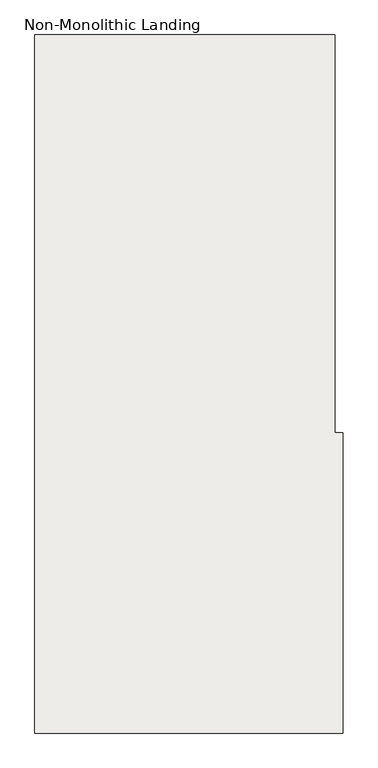
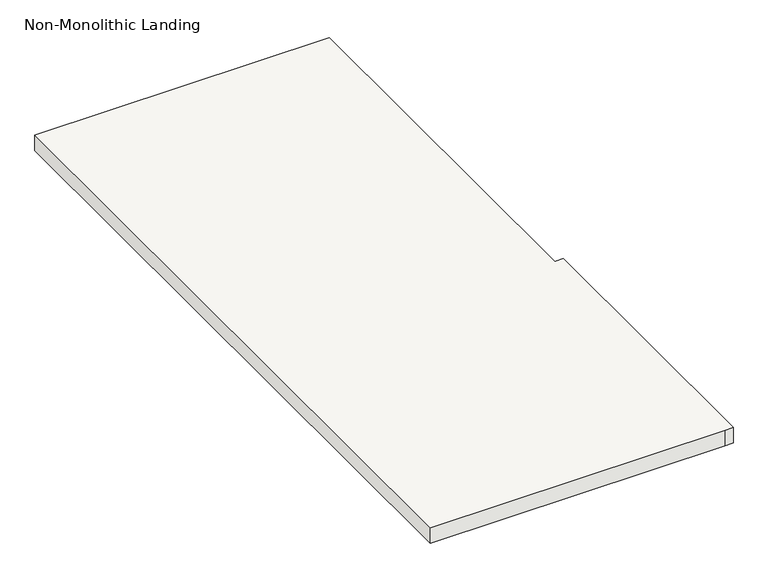
"""IFC4 building model written with IfcOpenShell, lengths in millimetres: slab geometry, Non-Monolithic Landing."""

from ifc_helpers import new_model, si_unit, origin, place, context, project, spatial, faceted_brep, source, transform, mapped, element, save


def non_monolithic_landing_459b2879(model_context):
    return source(origin(), model_context, "Body", "Brep", [
        faceted_brep([(-8810.2517085, 2919.0826226, 2123.0166667), (-8784.8517085, 2919.0826226, 2148.4166667), (-8784.8517085, 2004.6826226, 2148.4166667), (-8810.2517085, 2004.6826226, 2123.0166667), (-9699.2517085, 2919.0826226, 2167.4666667), (-9699.2517085, 792.0165128, 2167.4666667), (-8784.8517085, 792.0165128, 2167.4666667), (-8759.4517085, 792.0165128, 2167.4666667), (-8759.4517085, 1706.4165128, 2167.4666667), (-8784.8517085, 1706.4165128, 2167.4666667), (-8784.8517085, 2919.0826226, 2167.4666667), (-8810.2517085, 2004.6826226, 2116.6666667), (-8784.8517085, 2004.6826226, 2116.6666667), (-8784.8517085, 1706.4165128, 2116.6666667), (-8759.4517085, 1706.4165128, 2116.6666667), (-8759.4517085, 792.0165128, 2116.6666667), (-8784.8517085, 792.0165128, 2116.6666667), (-9699.2517085, 792.0165128, 2116.6666667), (-9699.2517085, 2919.0826226, 2116.6666667), (-8810.2517085, 2919.0826226, 2116.6666667)], [[[0, 1, 2, 3]], [[4, 5, 6, 7, 8, 9, 10]], [[11, 12, 13, 14, 15, 16, 17, 18, 19]], [[12, 11, 3, 2]], [[11, 19, 0, 3]], [[4, 10, 1, 0, 19, 18]], [[5, 4, 18, 17]], [[6, 5, 17, 16]], [[7, 6, 16, 15]], [[8, 7, 15, 14]], [[9, 8, 14, 13]], [[10, 9, 13, 12, 2, 1]]]),
    ])


if __name__ == "__main__":
    model = new_model("IFC4")
    model_context = context("Model", 3, world=origin())
    ifc_project = project(units=[si_unit("LENGTHUNIT", "METRE", prefix="MILLI")], contexts=[model_context])
    site = spatial("IfcSite", under=ifc_project)
    building = spatial("IfcBuilding", under=site)
    placement = place(None, origin())
    non_monolithic_landing_shape = non_monolithic_landing_459b2879(model_context)
    element("IfcSlab", 1, ObjectType="Non-Monolithic Landing", at=placement, inside=building, context=model_context, shape_type="MappedRepresentation", body=[
        mapped(non_monolithic_landing_shape, transform((0.0, 0.0, 0.0), x_axis=(1.0, 0.0, 0.0), y_axis=(0.0, 1.0, 0.0), z_axis=(0.0, 0.0, 1.0))),
    ])
    save(model, "model.ifc")
